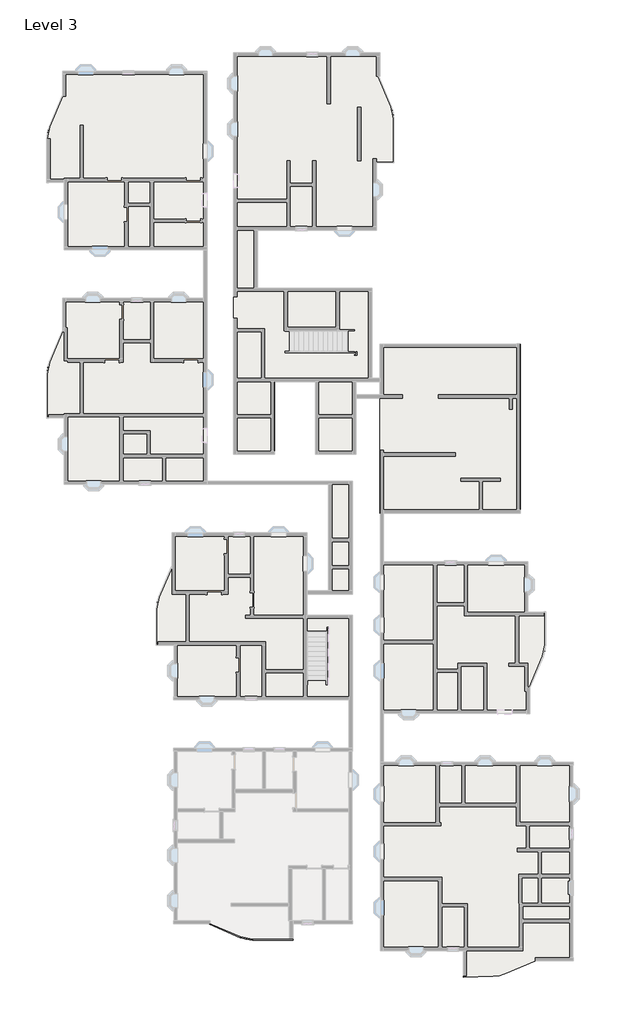
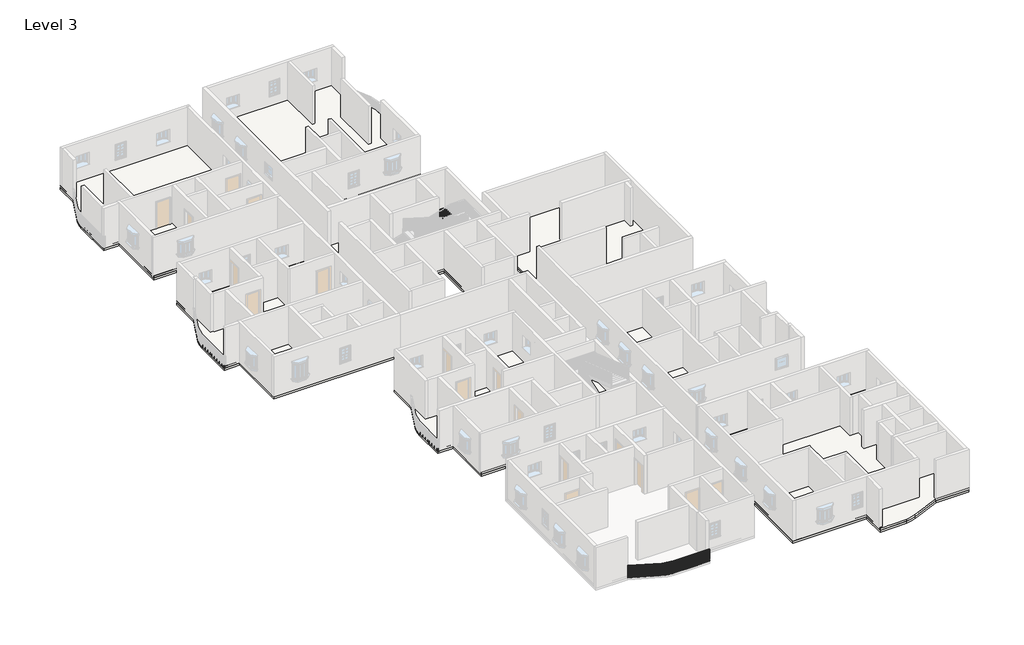
# One storey, part 5 of 14: 13 roofs, 12 slabs, 1 railing.
"""IFC4 building model written with IfcOpenShell, lengths in millimetres."""

from ifc_helpers import new_model, si_unit, point, frame, frame_2d, origin, place, context, project, spatial, polyline, circle_curve, trimmed, segment, composite_curve, outline, extrude, element, save
from ifc_brep_helpers import plane_surface, cylinder_surface, revolved_surface, advanced_brep

model = new_model("IFC4")

# Units and contexts
model_context = context("Model", 3, world=origin())
ifc_project = project(units=[si_unit("LENGTHUNIT", "METRE", prefix="MILLI")], contexts=[model_context])

# Site, building, storey
site = spatial("IfcSite", under=ifc_project)
building = spatial("IfcBuilding", under=site)
storey = spatial("IfcBuildingStorey", under=building, Name="Level 3", Elevation=6096.0)

# Railing
placement = place(None, origin())
element("IfcRailing", 1, ObjectType="Handrail - Rectangular", at=placement, inside=storey, context=model_context, shape_type="SolidModel", body=[
    advanced_brep(
    [(-10014.8722294, -25076.9923935, 7010.4), (-10014.8722294, -25076.9923935, 6959.6), (-10034.8694485, -25123.6909077, 6959.6), (-10034.8694485, -25123.6909077, 7010.4), (-8065.5370278, -25911.7359335, 7010.4), (-8065.5370278, -25911.7359335, 6959.6), (-8085.5342469, -25958.4344477, 6959.6), (-8085.5342469, -25958.4344477, 7010.4), (-7315.6413127, -26065.5416506, 6959.6), (-7315.6413127, -26065.5416506, 7010.4), (-7315.6413127, -26116.3416506, 6959.6), (-7315.6413127, -26116.3416506, 7010.4), (-4746.0891351, -26065.5416506, 7010.4), (-4746.0891351, -26116.3416506, 7010.4), (-4746.0891351, -26116.3416506, 6959.6), (-4746.0891351, -26065.5416506, 6959.6)],
    [
        (0, 1),
        (1, 2),
        (2, 3),
        (3, 0),
        (0, 4),
        (4, 5),
        (5, 1),
        (5, 6),
        (6, 2),
        (6, 7),
        (7, 3),
        (7, 4),
        (8, 5, circle_curve(frame((-7315.6413127, -24160.5416506, 6959.6), z_axis=(0.0, 0.0, -1.0), x_axis=(-0.3936460446736572, -0.9192620907623599, 0.0)), 1905.0)),
        (4, 9, circle_curve(frame((-7315.6413127, -24160.5416506, 7010.4), z_axis=(0.0, 0.0, 1.0), x_axis=(-0.3936460446736572, -0.9192620907623599, 0.0)), 1905.0)),
        (9, 8),
        (10, 6, circle_curve(frame((-7315.6413127, -24160.5416506, 6959.6), z_axis=(0.0, 0.0, -1.0), x_axis=(-0.3936460446736572, -0.9192620907623599, 0.0)), 1955.8)),
        (8, 10),
        (11, 7, circle_curve(frame((-7315.6413127, -24160.5416506, 7010.4), z_axis=(0.0, 0.0, -1.0), x_axis=(-0.3936460446736572, -0.9192620907623599, 0.0)), 1955.8)),
        (10, 11),
        (11, 9),
        (12, 13),
        (13, 14),
        (14, 15),
        (15, 12),
        (9, 12),
        (15, 8),
        (14, 10),
        (13, 11),
    ],
    [
        plane_surface(frame((-10024.8708389, -25100.3416506, 7010.4), z_axis=(-0.9192620907623597, 0.39364604467365766, 0.0), x_axis=(0.39364604467365766, 0.9192620907623597, 0.0))),
        plane_surface(frame((-10014.8722294, -25076.9923935, 7010.4), z_axis=(0.3936460446736571, 0.9192620907623599, 0.0), x_axis=(0.9192620907623599, -0.3936460446736571, 0.0))),
        plane_surface(frame((-10014.8722294, -25076.9923935, 6959.6), z_axis=(0.0, 0.0, -1.0), x_axis=(0.9192620907623599, -0.3936460446736571, 0.0))),
        plane_surface(frame((-10034.8694485, -25123.6909077, 6959.6), z_axis=(-0.3936460446736573, -0.9192620907623599, 0.0), x_axis=(0.9192620907623599, -0.3936460446736573, 0.0))),
        plane_surface(frame((-10034.8694485, -25123.6909077, 7010.4), z_axis=(0.0, 0.0, 1.0000000000000002), x_axis=(0.9192620907623599, -0.3936460446736573, 0.0))),
        revolved_surface(polyline([(-8065.537027803317, -25911.735933502296, 7010.4), (-8065.537027803317, -25911.735933502296, 6959.6)]), (-7315.6413127, -24160.5416506, 7010.4), (0.0, 0.0, 1.0)),
        plane_surface(frame((-7315.6413127, -24160.5416506, 6959.6), z_axis=(0.0, 0.0, -1.0), x_axis=(-0.3936460446736572, -0.9192620907623599, 0.0))),
        cylinder_surface(frame((-7315.6413127, -24160.5416506, 7010.4), z_axis=(0.0, 0.0, 1.0), x_axis=(-0.3936460446736572, -0.9192620907623599, 0.0)), 1955.8),
        plane_surface(frame((-7315.6413127, -24160.5416506, 7010.4), z_axis=(0.0, 0.0, 1.0), x_axis=(-0.3936460446736572, -0.9192620907623599, 0.0))),
        plane_surface(frame((-4746.0891351, -26090.9416506, 7010.4), z_axis=(1.0, 0.0, 0.0), x_axis=(0.0, 1.0, 0.0))),
        plane_surface(frame((-7315.6413127, -26065.5416506, 7010.4), z_axis=(0.0, 1.0, 0.0), x_axis=(1.0, 0.0, 0.0))),
        plane_surface(frame((-7315.6413127, -26065.5416506, 6959.6), z_axis=(0.0, 0.0, -1.0), x_axis=(1.0, 0.0, 0.0))),
        plane_surface(frame((-7315.6413127, -26116.3416506, 6959.6), z_axis=(0.0, -1.0, 0.0), x_axis=(1.0, 0.0, 0.0))),
        plane_surface(frame((-7315.6413127, -26116.3416506, 7010.4), z_axis=(0.0, 0.0, 1.0), x_axis=(1.0, 0.0, 0.0))),
    ],
    [
        (0, [[1, 2, 3, 4]]),
        (1, [[-1, 5, 6, 7]]),
        (2, [[-2, -7, 8, 9]]),
        (3, [[-3, -9, 10, 11]]),
        (4, [[-4, -11, 12, -5]]),
        (5, [[13, -6, 14, 15]]),
        (6, [[16, -8, -13, 17]]),
        (7, [[18, -10, -16, 19]]),
        (8, [[-14, -12, -18, 20]]),
        (9, [[21, 22, 23, 24]]),
        (10, [[-15, 25, -24, 26]]),
        (11, [[-17, -26, -23, 27]]),
        (12, [[-19, -27, -22, 28]]),
        (13, [[-20, -28, -21, -25]]),
    ],
),
    extrude(outline(polyline([(-4785.1663127, -26100.4666506), (-4785.1663127, -26081.4166506), (-4766.1163127, -26081.4166506), (-4766.1163127, -26100.4666506), (-4785.1663127, -26100.4666506)])), frame((0.0, 0.0, 6096.0), z_axis=(0.0, 0.0, 1.0), x_axis=(1.0, 0.0, 0.0)), (0.0, 0.0, 1.0), 863.6),
    extrude(outline(polyline([(-4886.7663127, -26100.4666506), (-4886.7663127, -26081.4166506), (-4867.7163127, -26081.4166506), (-4867.7163127, -26100.4666506), (-4886.7663127, -26100.4666506)])), frame((0.0, 0.0, 6096.0), z_axis=(0.0, 0.0, 1.0), x_axis=(1.0, 0.0, 0.0)), (0.0, 0.0, 1.0), 863.6),
    extrude(outline(polyline([(-4988.3663127, -26100.4666506), (-4988.3663127, -26081.4166506), (-4969.3163127, -26081.4166506), (-4969.3163127, -26100.4666506), (-4988.3663127, -26100.4666506)])), frame((0.0, 0.0, 6096.0), z_axis=(0.0, 0.0, 1.0), x_axis=(1.0, 0.0, 0.0)), (0.0, 0.0, 1.0), 863.6),
    extrude(outline(polyline([(-5089.9663127, -26100.4666506), (-5089.9663127, -26081.4166506), (-5070.9163127, -26081.4166506), (-5070.9163127, -26100.4666506), (-5089.9663127, -26100.4666506)])), frame((0.0, 0.0, 6096.0), z_axis=(0.0, 0.0, 1.0), x_axis=(1.0, 0.0, 0.0)), (0.0, 0.0, 1.0), 863.6),
    extrude(outline(polyline([(-5191.5663127, -26100.4666506), (-5191.5663127, -26081.4166506), (-5172.5163127, -26081.4166506), (-5172.5163127, -26100.4666506), (-5191.5663127, -26100.4666506)])), frame((0.0, 0.0, 6096.0), z_axis=(0.0, 0.0, 1.0), x_axis=(1.0, 0.0, 0.0)), (0.0, 0.0, 1.0), 863.6),
    extrude(outline(polyline([(-5293.1663127, -26100.4666506), (-5293.1663127, -26081.4166506), (-5274.1163127, -26081.4166506), (-5274.1163127, -26100.4666506), (-5293.1663127, -26100.4666506)])), frame((0.0, 0.0, 6096.0), z_axis=(0.0, 0.0, 1.0), x_axis=(1.0, 0.0, 0.0)), (0.0, 0.0, 1.0), 863.6),
    extrude(outline(polyline([(-5394.7663127, -26100.4666506), (-5394.7663127, -26081.4166506), (-5375.7163127, -26081.4166506), (-5375.7163127, -26100.4666506), (-5394.7663127, -26100.4666506)])), frame((0.0, 0.0, 6096.0), z_axis=(0.0, 0.0, 1.0), x_axis=(1.0, 0.0, 0.0)), (0.0, 0.0, 1.0), 863.6),
    extrude(outline(polyline([(-5496.3663127, -26100.4666506), (-5496.3663127, -26081.4166506), (-5477.3163127, -26081.4166506), (-5477.3163127, -26100.4666506), (-5496.3663127, -26100.4666506)])), frame((0.0, 0.0, 6096.0), z_axis=(0.0, 0.0, 1.0), x_axis=(1.0, 0.0, 0.0)), (0.0, 0.0, 1.0), 863.6),
    extrude(outline(polyline([(-5597.9663127, -26100.4666506), (-5597.9663127, -26081.4166506), (-5578.9163127, -26081.4166506), (-5578.9163127, -26100.4666506), (-5597.9663127, -26100.4666506)])), frame((0.0, 0.0, 6096.0), z_axis=(0.0, 0.0, 1.0), x_axis=(1.0, 0.0, 0.0)), (0.0, 0.0, 1.0), 863.6),
    extrude(outline(polyline([(-5699.5663127, -26100.4666506), (-5699.5663127, -26081.4166506), (-5680.5163127, -26081.4166506), (-5680.5163127, -26100.4666506), (-5699.5663127, -26100.4666506)])), frame((0.0, 0.0, 6096.0), z_axis=(0.0, 0.0, 1.0), x_axis=(1.0, 0.0, 0.0)), (0.0, 0.0, 1.0), 863.6),
    extrude(outline(polyline([(-5801.1663127, -26100.4666506), (-5801.1663127, -26081.4166506), (-5782.1163127, -26081.4166506), (-5782.1163127, -26100.4666506), (-5801.1663127, -26100.4666506)])), frame((0.0, 0.0, 6096.0), z_axis=(0.0, 0.0, 1.0), x_axis=(1.0, 0.0, 0.0)), (0.0, 0.0, 1.0), 863.6),
    extrude(outline(polyline([(-5902.7663127, -26100.4666506), (-5902.7663127, -26081.4166506), (-5883.7163127, -26081.4166506), (-5883.7163127, -26100.4666506), (-5902.7663127, -26100.4666506)])), frame((0.0, 0.0, 6096.0), z_axis=(0.0, 0.0, 1.0), x_axis=(1.0, 0.0, 0.0)), (0.0, 0.0, 1.0), 863.6),
    extrude(outline(polyline([(-6004.3663127, -26100.4666506), (-6004.3663127, -26081.4166506), (-5985.3163127, -26081.4166506), (-5985.3163127, -26100.4666506), (-6004.3663127, -26100.4666506)])), frame((0.0, 0.0, 6096.0), z_axis=(0.0, 0.0, 1.0), x_axis=(1.0, 0.0, 0.0)), (0.0, 0.0, 1.0), 863.6),
    extrude(outline(polyline([(-6105.9663127, -26100.4666506), (-6105.9663127, -26081.4166506), (-6086.9163127, -26081.4166506), (-6086.9163127, -26100.4666506), (-6105.9663127, -26100.4666506)])), frame((0.0, 0.0, 6096.0), z_axis=(0.0, 0.0, 1.0), x_axis=(1.0, 0.0, 0.0)), (0.0, 0.0, 1.0), 863.6),
    extrude(outline(polyline([(-6207.5663127, -26100.4666506), (-6207.5663127, -26081.4166506), (-6188.5163127, -26081.4166506), (-6188.5163127, -26100.4666506), (-6207.5663127, -26100.4666506)])), frame((0.0, 0.0, 6096.0), z_axis=(0.0, 0.0, 1.0), x_axis=(1.0, 0.0, 0.0)), (0.0, 0.0, 1.0), 863.6),
    extrude(outline(polyline([(-6309.1663127, -26100.4666506), (-6309.1663127, -26081.4166506), (-6290.1163127, -26081.4166506), (-6290.1163127, -26100.4666506), (-6309.1663127, -26100.4666506)])), frame((0.0, 0.0, 6096.0), z_axis=(0.0, 0.0, 1.0), x_axis=(1.0, 0.0, 0.0)), (0.0, 0.0, 1.0), 863.6),
    extrude(outline(polyline([(-6410.7663127, -26100.4666506), (-6410.7663127, -26081.4166506), (-6391.7163127, -26081.4166506), (-6391.7163127, -26100.4666506), (-6410.7663127, -26100.4666506)])), frame((0.0, 0.0, 6096.0), z_axis=(0.0, 0.0, 1.0), x_axis=(1.0, 0.0, 0.0)), (0.0, 0.0, 1.0), 863.6),
    extrude(outline(polyline([(-6512.3663127, -26100.4666506), (-6512.3663127, -26081.4166506), (-6493.3163127, -26081.4166506), (-6493.3163127, -26100.4666506), (-6512.3663127, -26100.4666506)])), frame((0.0, 0.0, 6096.0), z_axis=(0.0, 0.0, 1.0), x_axis=(1.0, 0.0, 0.0)), (0.0, 0.0, 1.0), 863.6),
    extrude(outline(polyline([(-6613.9663127, -26100.4666506), (-6613.9663127, -26081.4166506), (-6594.9163127, -26081.4166506), (-6594.9163127, -26100.4666506), (-6613.9663127, -26100.4666506)])), frame((0.0, 0.0, 6096.0), z_axis=(0.0, 0.0, 1.0), x_axis=(1.0, 0.0, 0.0)), (0.0, 0.0, 1.0), 863.6),
    extrude(outline(polyline([(-6715.5663127, -26100.4666506), (-6715.5663127, -26081.4166506), (-6696.5163127, -26081.4166506), (-6696.5163127, -26100.4666506), (-6715.5663127, -26100.4666506)])), frame((0.0, 0.0, 6096.0), z_axis=(0.0, 0.0, 1.0), x_axis=(1.0, 0.0, 0.0)), (0.0, 0.0, 1.0), 863.6),
    extrude(outline(polyline([(-6817.1663127, -26100.4666506), (-6817.1663127, -26081.4166506), (-6798.1163127, -26081.4166506), (-6798.1163127, -26100.4666506), (-6817.1663127, -26100.4666506)])), frame((0.0, 0.0, 6096.0), z_axis=(0.0, 0.0, 1.0), x_axis=(1.0, 0.0, 0.0)), (0.0, 0.0, 1.0), 863.6),
    extrude(outline(polyline([(-6918.7663127, -26100.4666506), (-6918.7663127, -26081.4166506), (-6899.7163127, -26081.4166506), (-6899.7163127, -26100.4666506), (-6918.7663127, -26100.4666506)])), frame((0.0, 0.0, 6096.0), z_axis=(0.0, 0.0, 1.0), x_axis=(1.0, 0.0, 0.0)), (0.0, 0.0, 1.0), 863.6),
    extrude(outline(polyline([(-7020.3663127, -26100.4666506), (-7020.3663127, -26081.4166506), (-7001.3163127, -26081.4166506), (-7001.3163127, -26100.4666506), (-7020.3663127, -26100.4666506)])), frame((0.0, 0.0, 6096.0), z_axis=(0.0, 0.0, 1.0), x_axis=(1.0, 0.0, 0.0)), (0.0, 0.0, 1.0), 863.6),
    extrude(outline(polyline([(-7121.9663127, -26100.4666506), (-7121.9663127, -26081.4166506), (-7102.9163127, -26081.4166506), (-7102.9163127, -26100.4666506), (-7121.9663127, -26100.4666506)])), frame((0.0, 0.0, 6096.0), z_axis=(0.0, 0.0, 1.0), x_axis=(1.0, 0.0, 0.0)), (0.0, 0.0, 1.0), 863.6),
    extrude(outline(polyline([(-7223.5663127, -26100.4666506), (-7223.5663127, -26081.4166506), (-7204.5163127, -26081.4166506), (-7204.5163127, -26100.4666506), (-7223.5663127, -26100.4666506)])), frame((0.0, 0.0, 6096.0), z_axis=(0.0, 0.0, 1.0), x_axis=(1.0, 0.0, 0.0)), (0.0, 0.0, 1.0), 863.6),
    extrude(outline(polyline([(-7395.3185803, -26098.8530973), (-7394.6296262, -26079.8155596), (-7375.5920885, -26080.5045137), (-7376.2810426, -26099.5420514), (-7395.3185803, -26098.8530973)])), frame((0.0, 0.0, 6096.0), z_axis=(0.0, 0.0, 1.0), x_axis=(1.0, 0.0, 0.0)), (0.0, 0.0, 1.0), 863.6),
    extrude(outline(polyline([(-7497.177549, -26091.9774704), (-7495.4880357, -26073.0025384), (-7476.5131037, -26074.6920517), (-7478.2026169, -26093.6669837), (-7497.177549, -26091.9774704)])), frame((0.0, 0.0, 6096.0), z_axis=(0.0, 0.0, 1.0), x_axis=(1.0, 0.0, 0.0)), (0.0, 0.0, 1.0), 863.6),
    extrude(outline(polyline([(-7598.5337632, -26079.7528408), (-7595.8483698, -26060.8930645), (-7576.9885935, -26063.5784579), (-7579.6739869, -26082.4382342), (-7598.5337632, -26079.7528408)])), frame((0.0, 0.0, 6096.0), z_axis=(0.0, 0.0, 1.0), x_axis=(1.0, 0.0, 0.0)), (0.0, 0.0, 1.0), 863.6),
    extrude(outline(polyline([(-7699.1065227, -26062.2130639), (-7695.4326862, -26043.5206744), (-7676.7402967, -26047.1945108), (-7680.4141332, -26065.8869003), (-7699.1065227, -26062.2130639)])), frame((0.0, 0.0, 6096.0), z_axis=(0.0, 0.0, 1.0), x_axis=(1.0, 0.0, 0.0)), (0.0, 0.0, 1.0), 863.6),
    extrude(outline(polyline([(-7798.6172969, -26039.4067149), (-7793.9651918, -26020.9334797), (-7775.4919566, -26025.5855848), (-7780.1440617, -26044.05882), (-7798.6172969, -26039.4067149)])), frame((0.0, 0.0, 6096.0), z_axis=(0.0, 0.0, 1.0), x_axis=(1.0, 0.0, 0.0)), (0.0, 0.0, 1.0), 863.6),
    extrude(outline(polyline([(-7896.7904963, -26011.396955), (-7891.1730064, -25993.1940347), (-7872.9700861, -25998.8115246), (-7878.587576, -26017.0144449), (-7896.7904963, -26011.396955)])), frame((0.0, 0.0, 6096.0), z_axis=(0.0, 0.0, 1.0), x_axis=(1.0, 0.0, 0.0)), (0.0, 0.0, 1.0), 863.6),
    extrude(outline(polyline([(-7993.3542357, -25978.2613554), (-7986.7869183, -25960.379162), (-7968.9047249, -25966.9464794), (-7975.4720423, -25984.8286729), (-7993.3542357, -25978.2613554)])), frame((0.0, 0.0, 6096.0), z_axis=(0.0, 0.0, 1.0), x_axis=(1.0, 0.0, 0.0)), (0.0, 0.0, 1.0), 863.6),
    extrude(outline(polyline([(-8169.4357205, -25905.2369062), (-8161.9367633, -25887.7249634), (-8144.4248205, -25895.2239205), (-8151.9237777, -25912.7358634), (-8169.4357205, -25905.2369062)])), frame((0.0, 0.0, 6096.0), z_axis=(0.0, 0.0, 1.0), x_axis=(1.0, 0.0, 0.0)), (0.0, 0.0, 1.0), 863.6),
    extrude(outline(polyline([(-8262.8327489, -25865.2424681), (-8255.3337918, -25847.7305252), (-8237.8218489, -25855.2294824), (-8245.3208061, -25872.7414252), (-8262.8327489, -25865.2424681)])), frame((0.0, 0.0, 6096.0), z_axis=(0.0, 0.0, 1.0), x_axis=(1.0, 0.0, 0.0)), (0.0, 0.0, 1.0), 863.6),
    extrude(outline(polyline([(-8356.2297773, -25825.2480299), (-8348.7308202, -25807.7360871), (-8331.2188774, -25815.2350443), (-8338.7178345, -25832.7469871), (-8356.2297773, -25825.2480299)])), frame((0.0, 0.0, 6096.0), z_axis=(0.0, 0.0, 1.0), x_axis=(1.0, 0.0, 0.0)), (0.0, 0.0, 1.0), 863.6),
    extrude(outline(polyline([(-8449.6268058, -25785.2535918), (-8442.1278486, -25767.741649), (-8424.6159058, -25775.2406061), (-8432.1148629, -25792.752549), (-8449.6268058, -25785.2535918)])), frame((0.0, 0.0, 6096.0), z_axis=(0.0, 0.0, 1.0), x_axis=(1.0, 0.0, 0.0)), (0.0, 0.0, 1.0), 863.6),
    extrude(outline(polyline([(-8543.0238342, -25745.2591537), (-8535.524877, -25727.7472108), (-8518.0129342, -25735.246168), (-8525.5118914, -25752.7581108), (-8543.0238342, -25745.2591537)])), frame((0.0, 0.0, 6096.0), z_axis=(0.0, 0.0, 1.0), x_axis=(1.0, 0.0, 0.0)), (0.0, 0.0, 1.0), 863.6),
    extrude(outline(polyline([(-8636.4208626, -25705.2647155), (-8628.9219055, -25687.7527727), (-8611.4099626, -25695.2517298), (-8618.9089198, -25712.7636727), (-8636.4208626, -25705.2647155)])), frame((0.0, 0.0, 6096.0), z_axis=(0.0, 0.0, 1.0), x_axis=(1.0, 0.0, 0.0)), (0.0, 0.0, 1.0), 863.6),
    extrude(outline(polyline([(-8729.817891, -25665.2702774), (-8722.3189339, -25647.7583346), (-8704.806991, -25655.2572917), (-8712.3059482, -25672.7692345), (-8729.817891, -25665.2702774)])), frame((0.0, 0.0, 6096.0), z_axis=(0.0, 0.0, 1.0), x_axis=(1.0, 0.0, 0.0)), (0.0, 0.0, 1.0), 863.6),
    extrude(outline(polyline([(-8823.2149194, -25625.2758392), (-8815.7159623, -25607.7638964), (-8798.2040195, -25615.2628536), (-8805.7029766, -25632.7747964), (-8823.2149194, -25625.2758392)])), frame((0.0, 0.0, 6096.0), z_axis=(0.0, 0.0, 1.0), x_axis=(1.0, 0.0, 0.0)), (0.0, 0.0, 1.0), 863.6),
    extrude(outline(polyline([(-8916.6119479, -25585.2814011), (-8909.1129907, -25567.7694583), (-8891.6010479, -25575.2684154), (-8899.100005, -25592.7803583), (-8916.6119479, -25585.2814011)])), frame((0.0, 0.0, 6096.0), z_axis=(0.0, 0.0, 1.0), x_axis=(1.0, 0.0, 0.0)), (0.0, 0.0, 1.0), 863.6),
    extrude(outline(polyline([(-9010.0089763, -25545.286963), (-9002.5100191, -25527.7750201), (-8984.9980763, -25535.2739773), (-8992.4970335, -25552.7859201), (-9010.0089763, -25545.286963)])), frame((0.0, 0.0, 6096.0), z_axis=(0.0, 0.0, 1.0), x_axis=(1.0, 0.0, 0.0)), (0.0, 0.0, 1.0), 863.6),
    extrude(outline(polyline([(-9103.4060047, -25505.2925248), (-9095.9070476, -25487.780582), (-9078.3951047, -25495.2795391), (-9085.8940619, -25512.791482), (-9103.4060047, -25505.2925248)])), frame((0.0, 0.0, 6096.0), z_axis=(0.0, 0.0, 1.0), x_axis=(1.0, 0.0, 0.0)), (0.0, 0.0, 1.0), 863.6),
    extrude(outline(polyline([(-9196.8030331, -25465.2980867), (-9189.304076, -25447.7861439), (-9171.7921332, -25455.285101), (-9179.2910903, -25472.7970438), (-9196.8030331, -25465.2980867)])), frame((0.0, 0.0, 6096.0), z_axis=(0.0, 0.0, 1.0), x_axis=(1.0, 0.0, 0.0)), (0.0, 0.0, 1.0), 863.6),
    extrude(outline(polyline([(-9290.2000616, -25425.3036485), (-9282.7011044, -25407.7917057), (-9265.1891616, -25415.2906629), (-9272.6881187, -25432.8026057), (-9290.2000616, -25425.3036485)])), frame((0.0, 0.0, 6096.0), z_axis=(0.0, 0.0, 1.0), x_axis=(1.0, 0.0, 0.0)), (0.0, 0.0, 1.0), 863.6),
    extrude(outline(polyline([(-9383.59709, -25385.3092104), (-9376.0981328, -25367.7972676), (-9358.58619, -25375.2962247), (-9366.0851471, -25392.8081676), (-9383.59709, -25385.3092104)])), frame((0.0, 0.0, 6096.0), z_axis=(0.0, 0.0, 1.0), x_axis=(1.0, 0.0, 0.0)), (0.0, 0.0, 1.0), 863.6),
    extrude(outline(polyline([(-9476.9941184, -25345.3147723), (-9469.4951612, -25327.8028294), (-9451.9832184, -25335.3017866), (-9459.4821756, -25352.8137294), (-9476.9941184, -25345.3147723)])), frame((0.0, 0.0, 6096.0), z_axis=(0.0, 0.0, 1.0), x_axis=(1.0, 0.0, 0.0)), (0.0, 0.0, 1.0), 863.6),
    extrude(outline(polyline([(-9570.3911468, -25305.3203341), (-9562.8921897, -25287.8083913), (-9545.3802468, -25295.3073485), (-9552.879204, -25312.8192913), (-9570.3911468, -25305.3203341)])), frame((0.0, 0.0, 6096.0), z_axis=(0.0, 0.0, 1.0), x_axis=(1.0, 0.0, 0.0)), (0.0, 0.0, 1.0), 863.6),
    extrude(outline(polyline([(-9663.7881752, -25265.325896), (-9656.2892181, -25247.8139532), (-9638.7772753, -25255.3129103), (-9646.2762324, -25272.8248531), (-9663.7881752, -25265.325896)])), frame((0.0, 0.0, 6096.0), z_axis=(0.0, 0.0, 1.0), x_axis=(1.0, 0.0, 0.0)), (0.0, 0.0, 1.0), 863.6),
    extrude(outline(polyline([(-9757.1852037, -25225.3314579), (-9749.6862465, -25207.819515), (-9732.1743037, -25215.3184722), (-9739.6732608, -25232.830415), (-9757.1852037, -25225.3314579)])), frame((0.0, 0.0, 6096.0), z_axis=(0.0, 0.0, 1.0), x_axis=(1.0, 0.0, 0.0)), (0.0, 0.0, 1.0), 863.6),
    extrude(outline(polyline([(-9850.5822321, -25185.3370197), (-9843.0832749, -25167.8250769), (-9825.5713321, -25175.324034), (-9833.0702893, -25192.8359769), (-9850.5822321, -25185.3370197)])), frame((0.0, 0.0, 6096.0), z_axis=(0.0, 0.0, 1.0), x_axis=(1.0, 0.0, 0.0)), (0.0, 0.0, 1.0), 863.6),
    extrude(outline(polyline([(-9943.9792605, -25145.3425816), (-9936.4803034, -25127.8306387), (-9918.9683605, -25135.3295959), (-9926.4673177, -25152.8415387), (-9943.9792605, -25145.3425816)])), frame((0.0, 0.0, 6096.0), z_axis=(0.0, 0.0, 1.0), x_axis=(1.0, 0.0, 0.0)), (0.0, 0.0, 1.0), 863.6),
    extrude(outline(polyline([(-7325.1663127, -26100.4666506), (-7325.1663127, -26081.4166506), (-7306.1163127, -26081.4166506), (-7306.1163127, -26100.4666506), (-7325.1663127, -26100.4666506)])), frame((0.0, 0.0, 6096.0), z_axis=(0.0, 0.0, 1.0), x_axis=(1.0, 0.0, 0.0)), (0.0, 0.0, 1.0), 863.6),
    extrude(outline(polyline([(-8088.0410874, -25940.0916834), (-8080.5421302, -25922.5797406), (-8063.0301874, -25930.0786978), (-8070.5291445, -25947.5906406), (-8088.0410874, -25940.0916834)])), frame((0.0, 0.0, 6096.0), z_axis=(0.0, 0.0, 1.0), x_axis=(1.0, 0.0, 0.0)), (0.0, 0.0, 1.0), 863.6),
    extrude(outline(polyline([(-4765.1391351, -26100.4666506), (-4765.1391351, -26081.4166506), (-4746.0891351, -26081.4166506), (-4746.0891351, -26100.4666506), (-4765.1391351, -26100.4666506)])), frame((0.0, 0.0, 6096.0), z_axis=(0.0, 0.0, 1.0), x_axis=(1.0, 0.0, 0.0)), (0.0, 0.0, 1.0), 863.6),
    extrude(outline(polyline([(-10028.6203175, -25109.097622), (-10021.1213604, -25091.5856792), (-10003.6094175, -25099.0846363), (-10011.1083747, -25116.5965792), (-10028.6203175, -25109.097622)])), frame((0.0, 0.0, 6096.0), z_axis=(0.0, 0.0, 1.0), x_axis=(1.0, 0.0, 0.0)), (0.0, 0.0, 1.0), 863.6),
])

# Roofs
element("IfcRoof", 2, ObjectType="Generic - 12\"", at=placement, inside=storey, context=model_context, shape_type="SweptSolid", body=[
    extrude(outline(composite_curve([segment(polyline([(6070.4380523, -26783.9042694), (812.6380523, -26783.9042694), (812.6380523, -14845.9042694), (13017.3380523, -14845.9042694), (13017.3380523, -27431.6042694), (10660.5280667, -27431.6042694), (8711.1928652, -28266.3478094)]), True, "CONTINUOUS"), segment(trimmed(circle_curve(frame_2d((7951.2985405, -26491.8042694)), 1930.4), [point((8711.1928652, -28266.3478094))], [point((7953.0959373, -28422.2034326))], False, "CARTESIAN"), True, "CONTINUOUS"), segment(polyline([(7953.0959373, -28422.2034326), (6070.4380523, -28487.9472947), (6070.4380523, -26783.9042694)]), True, "CONTINUOUS")], self_intersect=False)), frame((0.0, 0.0, 6096.0), z_axis=(0.0, 0.0, 1.0), x_axis=(1.0, 0.0, 0.0)), (0.0, 0.0, 1.0), 152.4),
])
element("IfcRoof", 3, ObjectType="Generic - 12\"", at=placement, inside=storey, context=model_context, shape_type="SweptSolid", body=[
    extrude(outline(composite_curve([segment(polyline([(10274.1380523, -11759.8042694), (803.8108649, -11759.8042694), (803.8108649, -2133.2042694), (10159.8380523, -2133.2042694), (10159.8380523, -5352.6542694), (11264.7380523, -5352.6542694), (11264.7380523, -7397.5810633)]), True, "CONTINUOUS"), segment(trimmed(circle_curve(frame_2d((9334.3380523, -7397.5810633)), 1930.4), [point((11264.7380523, -7397.5810633))], [point((11108.8815923, -8157.475388))], False, "CARTESIAN"), True, "CONTINUOUS"), segment(polyline([(11108.8815923, -8157.475388), (10274.1380523, -10106.8105895), (10274.1380523, -11759.8042694)]), True, "CONTINUOUS")], self_intersect=False)), frame((0.0, 0.0, 6096.0), z_axis=(0.0, 0.0, 1.0), x_axis=(1.0, 0.0, 0.0)), (0.0, 0.0, 1.0), 152.4),
])
element("IfcRoof", 4, ObjectType="Generic - 12\"", at=placement, inside=storey, context=model_context, shape_type="SweptSolid", body=[
    extrude(outline(composite_curve([segment(polyline([(-13395.387215, -7421.9416506), (-13395.387215, -5140.4900045)]), True, "CONTINUOUS"), segment(trimmed(circle_curve(frame_2d((-11464.987215, -5140.4900045)), 1930.4), [point((-13395.387215, -5140.4900045))], [point((-13239.530755, -4380.5956799))], False, "CARTESIAN"), True, "CONTINUOUS"), segment(polyline([(-13239.530755, -4380.5956799), (-12404.787215, -2431.2604783), (-12404.787215, -322.6416506), (-3857.687215, -322.6416506), (-3857.687215, -5523.2916506), (-974.1891351, -5523.2916506), (-974.1891351, -10889.0416506), (-12290.487215, -10889.0416506), (-12290.487215, -7421.9416506), (-13395.387215, -7421.9416506)]), True, "CONTINUOUS")], self_intersect=False)), frame((0.0, 0.0, 6096.0), z_axis=(0.0, 0.0, 1.0), x_axis=(1.0, 0.0, 0.0)), (0.0, 0.0, 1.0), 152.4),
])
element("IfcRoof", 5, ObjectType="Generic - 12\"", at=placement, inside=storey, context=model_context, shape_type="SweptSolid", body=[
    extrude(outline(polyline([(-2472.7891351, 2953.9583494), (-961.4891351, 2953.9583494), (-961.4891351, -4202.4916506), (-2472.7891351, -4202.4916506), (-2472.7891351, 2953.9583494)])), frame((0.0, 0.0, 6096.0), z_axis=(0.0, 0.0, 1.0), x_axis=(1.0, 0.0, 0.0)), (0.0, 0.0, 1.0), 152.4),
])
element("IfcRoof", 6, ObjectType="Generic - 12\"", at=placement, inside=storey, context=model_context, shape_type="SweptSolid", body=[
    extrude(outline(composite_curve([segment(polyline([(-10194.3891351, 2750.7583494), (-19236.7891351, 2750.7583494), (-19236.7891351, 6979.8583494), (-20341.6891351, 6979.8583494), (-20341.6891351, 9746.7948172)]), True, "CONTINUOUS"), segment(trimmed(circle_curve(frame_2d((-18411.2891351, 9746.7948172)), 1930.4), [point((-20341.6891351, 9746.7948172))], [point((-20185.8326751, 10506.6891419))], False, "CARTESIAN"), True, "CONTINUOUS"), segment(polyline([(-20185.8326751, 10506.6891419), (-19351.0891351, 12456.0243434), (-19351.0891351, 14536.3583494), (-10194.3891351, 14536.3583494), (-10194.3891351, 2750.7583494)]), True, "CONTINUOUS")], self_intersect=False)), frame((0.0, 0.0, 6096.0), z_axis=(0.0, 0.0, 1.0), x_axis=(1.0, 0.0, 0.0)), (0.0, 0.0, 1.0), 152.4),
])
element("IfcRoof", 7, ObjectType="Generic - 12\"", at=placement, inside=storey, context=model_context, shape_type="SweptSolid", body=[
    extrude(outline(composite_curve([segment(polyline([(-10194.3891351, 17609.7583494), (-19236.7891351, 17609.7583494), (-19236.7891351, 21889.6583494), (-20341.6891351, 21889.6583494), (-20341.6891351, 24656.5948172)]), True, "CONTINUOUS"), segment(trimmed(circle_curve(frame_2d((-18411.2891351, 24656.5948172)), 1930.4), [point((-20341.6891351, 24656.5948172))], [point((-20185.8326751, 25416.4891419))], False, "CARTESIAN"), True, "CONTINUOUS"), segment(polyline([(-20185.8326751, 25416.4891419), (-19351.0891351, 27365.8243434), (-19351.0891351, 28950.8583494), (-10194.3891351, 28950.8583494), (-10194.3891351, 17609.7583494)]), True, "CONTINUOUS")], self_intersect=False)), frame((0.0, 0.0, 6096.0), z_axis=(0.0, 0.0, 1.0), x_axis=(1.0, 0.0, 0.0)), (0.0, 0.0, 1.0), 152.4),
])
element("IfcRoof", 8, ObjectType="Generic - 12\"", at=placement, inside=storey, context=model_context, shape_type="SweptSolid", body=[
    extrude(outline(composite_curve([segment(polyline([(-8492.5891351, 18875.1215905), (-8492.5891351, 30101.9215905), (664.1108649, 30101.9215905), (664.1108649, 28631.1875845), (1498.8544049, 26681.8523829)]), True, "CONTINUOUS"), segment(trimmed(circle_curve(frame_2d((-275.6891351, 25921.9580583)), 1930.4), [point((1498.8544049, 26681.8523829))], [point((1654.7108649, 25921.9580583))], False, "CARTESIAN"), True, "CONTINUOUS"), segment(polyline([(1654.7108649, 25921.9580583), (1654.7108649, 23155.0215905), (549.8108649, 23155.0215905), (549.8108649, 18875.1215905), (-8492.5891351, 18875.1215905)]), True, "CONTINUOUS")], self_intersect=False)), frame((0.0, 0.0, 6096.0), z_axis=(0.0, 0.0, 1.0), x_axis=(1.0, 0.0, 0.0)), (0.0, 0.0, 1.0), 152.4),
])
element("IfcRoof", 9, ObjectType="Generic - 12\"", at=placement, inside=storey, context=model_context, shape_type="SweptSolid", body=[
    extrude(outline(polyline([(-8492.5891351, 9478.4949943), (-5914.4891351, 9478.4949943), (-5914.4891351, 4665.1949943), (-8492.5891351, 4665.1949943), (-8492.5891351, 9478.4949943)])), frame((0.0, 0.0, 6096.0), z_axis=(0.0, 0.0, 1.0), x_axis=(1.0, 0.0, 0.0)), (0.0, 0.0, 1.0), 152.4),
])
element("IfcRoof", 10, ObjectType="Generic - 12\"", at=placement, inside=storey, context=model_context, shape_type="SweptSolid", body=[
    extrude(outline(polyline([(-3310.9891351, 9478.4949943), (-745.5891351, 9478.4949943), (-745.5891351, 4652.4949943), (-3310.9891351, 4652.4949943), (-3310.9891351, 9478.4949943)])), frame((0.0, 0.0, 6096.0), z_axis=(0.0, 0.0, 1.0), x_axis=(1.0, 0.0, 0.0)), (0.0, 0.0, 1.0), 152.4),
])
element("IfcRoof", 11, ObjectType="Generic - 12\"", at=placement, inside=storey, context=model_context, shape_type="SweptSolid", body=[
    extrude(outline(polyline([(-8492.5891351, 19078.3215905), (-6993.9891351, 19078.3215905), (-6993.9891351, 14988.9215905), (-8492.5891351, 14988.9215905), (-8492.5891351, 19078.3215905)])), frame((0.0, 0.0, 6096.0), z_axis=(0.0, 0.0, 1.0), x_axis=(1.0, 0.0, 0.0)), (0.0, 0.0, 1.0), 152.4),
])
element("IfcRoof", 12, ObjectType="Generic - 12\"", at=placement, inside=storey, context=model_context, shape_type="SweptSolid", body=[
    extrude(outline(polyline([(-8492.5891351, 15192.1215905), (257.7108649, 15192.1215905), (257.7108649, 9275.2949943), (-8492.5891351, 9275.2949943), (-8492.5891351, 15192.1215905)])), frame((0.0, 0.0, 6096.0), z_axis=(0.0, 0.0, 1.0), x_axis=(1.0, 0.0, 0.0)), (0.0, 0.0, 1.0), 152.4),
])
element("IfcRoof", 13, ObjectType="Generic - 12\"", at=placement, inside=storey, context=model_context, shape_type="SweptSolid", body=[
    extrude(outline(polyline([(793.5880523, 11646.2957306), (9677.2380523, 11646.2957306), (9677.2380523, 940.1957306), (793.5880523, 940.1957306), (793.5880523, 11646.2957306)])), frame((0.0, 0.0, 6096.0), z_axis=(0.0, 0.0, 1.0), x_axis=(1.0, 0.0, 0.0)), (0.0, 0.0, 1.0), 152.4),
])
element("IfcRoof", 14, ObjectType="Generic - 12\"", at=placement, inside=storey, context=model_context, shape_type="SweptSolid", body=[
    extrude(outline(composite_curve([segment(polyline([(-8492.5891351, 18875.1215905), (-8492.5891351, 30101.9215905), (664.1108649, 30101.9215905), (664.1108649, 28631.1875845), (1498.8544049, 26681.8523829)]), True, "CONTINUOUS"), segment(trimmed(circle_curve(frame_2d((-275.6891351, 25921.9580583)), 1930.4), [point((1498.8544049, 26681.8523829))], [point((1654.7108649, 25921.9580583))], False, "CARTESIAN"), True, "CONTINUOUS"), segment(polyline([(1654.7108649, 25921.9580583), (1654.7108649, 23155.0215905), (549.8108649, 23155.0215905), (549.8108649, 18875.1215905), (-8492.5891351, 18875.1215905)]), True, "CONTINUOUS")], self_intersect=False)), frame((0.0, 0.0, 6096.0), z_axis=(0.0, 0.0, 1.0), x_axis=(1.0, 0.0, 0.0)), (0.0, 0.0, 1.0), 152.4),
])

# Slabs
element("IfcSlab", 15, ObjectType="Generic - 12\"", at=placement, inside=storey, context=model_context, shape_type="SweptSolid", body=[
    extrude(outline(composite_curve([segment(polyline([(-20341.6891351, 21889.6583494), (-20341.6891351, 24656.5948172)]), True, "CONTINUOUS"), segment(trimmed(circle_curve(frame_2d((-18411.2891351, 24656.5948172)), 1930.4), [point((-20341.6891351, 24656.5948172))], [point((-20185.8326751, 25416.4891419))], False, "CARTESIAN"), True, "CONTINUOUS"), segment(polyline([(-20185.8326751, 25416.4891419), (-19351.0891351, 27365.8243434), (-19351.0891351, 28950.8583494), (-10194.3891351, 28950.8583494), (-10194.3891351, 17609.7583494), (-19236.7891351, 17609.7583494), (-19236.7891351, 21889.6583494), (-20341.6891351, 21889.6583494)]), True, "CONTINUOUS")], self_intersect=False)), frame((0.0, 0.0, 5943.6), z_axis=(0.0, 0.0, 1.0), x_axis=(1.0, 0.0, 0.0)), (0.0, 0.0, 1.0), 152.4),
])
element("IfcSlab", 16, ObjectType="Generic - 12\"", at=placement, inside=storey, context=model_context, shape_type="SweptSolid", body=[
    extrude(outline(composite_curve([segment(polyline([(13017.3380523, -27431.6042694), (10660.5280667, -27431.6042694), (8711.1928652, -28266.3478094)]), True, "CONTINUOUS"), segment(trimmed(circle_curve(frame_2d((7951.2985405, -26491.8042694)), 1930.4), [point((8711.1928652, -28266.3478094))], [point((7953.0959373, -28422.2034326))], False, "CARTESIAN"), True, "CONTINUOUS"), segment(polyline([(7953.0959373, -28422.2034326), (6070.4380523, -28487.9472947), (6070.4380523, -26783.9042694), (812.6380523, -26783.9042694), (812.6380523, -14845.9042694), (13017.3380523, -14845.9042694), (13017.3380523, -27431.6042694)]), True, "CONTINUOUS")], self_intersect=False)), frame((0.0, 0.0, 5943.6), z_axis=(0.0, 0.0, 1.0), x_axis=(1.0, 0.0, 0.0)), (0.0, 0.0, 1.0), 152.4),
])
element("IfcSlab", 17, ObjectType="Generic - 12\"", at=placement, inside=storey, context=model_context, shape_type="SweptSolid", body=[
    extrude(outline(composite_curve([segment(polyline([(10274.1380523, -11759.8042694), (803.8108649, -11759.8042694), (803.8108649, -2133.2042694), (10159.8380523, -2133.2042694), (10159.8380523, -5352.6542694), (11264.7380523, -5352.6542694), (11264.7380523, -7397.5810633)]), True, "CONTINUOUS"), segment(trimmed(circle_curve(frame_2d((9334.3380523, -7397.5810633)), 1930.4), [point((11264.7380523, -7397.5810633))], [point((11108.8815923, -8157.475388))], False, "CARTESIAN"), True, "CONTINUOUS"), segment(polyline([(11108.8815923, -8157.475388), (10274.1380523, -10106.8105895), (10274.1380523, -11759.8042694)]), True, "CONTINUOUS")], self_intersect=False)), frame((0.0, 0.0, 5943.6), z_axis=(0.0, 0.0, 1.0), x_axis=(1.0, 0.0, 0.0)), (0.0, 0.0, 1.0), 152.4),
])
element("IfcSlab", 18, ObjectType="Generic - 12\"", at=placement, inside=storey, context=model_context, shape_type="SweptSolid", body=[
    extrude(outline(composite_curve([segment(polyline([(-974.1891351, -10889.0416506), (-12290.487215, -10889.0416506), (-12290.487215, -7421.9416506), (-13395.387215, -7421.9416506), (-13395.387215, -5140.4900045)]), True, "CONTINUOUS"), segment(trimmed(circle_curve(frame_2d((-11464.987215, -5140.4900045)), 1930.4), [point((-13395.387215, -5140.4900045))], [point((-13239.530755, -4380.5956799))], False, "CARTESIAN"), True, "CONTINUOUS"), segment(polyline([(-13239.530755, -4380.5956799), (-12404.787215, -2431.2604783), (-12404.787215, -322.6416506), (-3857.687215, -322.6416506), (-3857.687215, -5523.2916506), (-974.1891351, -5523.2916506), (-974.1891351, -10889.0416506)]), True, "CONTINUOUS")], self_intersect=False)), frame((0.0, 0.0, 5943.6), z_axis=(0.0, 0.0, 1.0), x_axis=(1.0, 0.0, 0.0)), (0.0, 0.0, 1.0), 152.4),
])
element("IfcSlab", 19, ObjectType="Generic - 12\"", at=placement, inside=storey, context=model_context, shape_type="SweptSolid", body=[
    extrude(outline(composite_curve([segment(polyline([(-20341.6891351, 6979.8583494), (-20341.6891351, 9746.7948172)]), True, "CONTINUOUS"), segment(trimmed(circle_curve(frame_2d((-18411.2891351, 9746.7948172)), 1930.4), [point((-20341.6891351, 9746.7948172))], [point((-20185.8326751, 10506.6891419))], False, "CARTESIAN"), True, "CONTINUOUS"), segment(polyline([(-20185.8326751, 10506.6891419), (-19351.0891351, 12456.0243434), (-19351.0891351, 14536.3583494), (-10194.3891351, 14536.3583494), (-10194.3891351, 2750.7583494), (-19236.7891351, 2750.7583494), (-19236.7891351, 6979.8583494), (-20341.6891351, 6979.8583494)]), True, "CONTINUOUS")], self_intersect=False)), frame((0.0, 0.0, 5943.6), z_axis=(0.0, 0.0, 1.0), x_axis=(1.0, 0.0, 0.0)), (0.0, 0.0, 1.0), 152.4),
])
element("IfcSlab", 20, ObjectType="Generic - 12\"", at=placement, inside=storey, context=model_context, shape_type="SweptSolid", body=[
    extrude(outline(composite_curve([segment(polyline([(549.8108649, 18875.1215905), (-8492.5891351, 18875.1215905), (-8492.5891351, 30101.9215905), (664.1108649, 30101.9215905), (664.1108649, 28631.1875845), (1498.8544049, 26681.8523829)]), True, "CONTINUOUS"), segment(trimmed(circle_curve(frame_2d((-275.6891351, 25921.9580583)), 1930.4), [point((1498.8544049, 26681.8523829))], [point((1654.7108649, 25921.9580583))], False, "CARTESIAN"), True, "CONTINUOUS"), segment(polyline([(1654.7108649, 25921.9580583), (1654.7108649, 23155.0215905), (549.8108649, 23155.0215905), (549.8108649, 18875.1215905)]), True, "CONTINUOUS")], self_intersect=False)), frame((0.0, 0.0, 5943.6), z_axis=(0.0, 0.0, 1.0), x_axis=(1.0, 0.0, 0.0)), (0.0, 0.0, 1.0), 152.4),
])
element("IfcSlab", 21, ObjectType="Generic - 12\"", at=placement, inside=storey, context=model_context, shape_type="SweptSolid", body=[
    extrude(outline(polyline([(257.7108649, 15192.1215905), (257.7108649, 9275.2949943), (-8492.5891351, 9275.2949943), (-8492.5891351, 15192.1215905), (257.7108649, 15192.1215905)])), frame((0.0, 0.0, 5943.6), z_axis=(0.0, 0.0, 1.0), x_axis=(1.0, 0.0, 0.0)), (0.0, 0.0, 1.0), 152.4),
])
element("IfcSlab", 22, ObjectType="Generic - 12\"", at=placement, inside=storey, context=model_context, shape_type="SweptSolid", body=[
    extrude(outline(polyline([(9677.2380523, 11646.2957306), (9677.2380523, 940.1957306), (793.5880523, 940.1957306), (793.5880523, 11646.2957306), (9677.2380523, 11646.2957306)])), frame((0.0, 0.0, 5943.6), z_axis=(0.0, 0.0, 1.0), x_axis=(1.0, 0.0, 0.0)), (0.0, 0.0, 1.0), 152.4),
])
element("IfcSlab", 23, ObjectType="Generic - 12\"", at=placement, inside=storey, context=model_context, shape_type="SweptSolid", body=[
    extrude(outline(polyline([(-5914.4891351, 9478.4949943), (-5914.4891351, 4665.1949943), (-8492.5891351, 4665.1949943), (-8492.5891351, 9478.4949943), (-5914.4891351, 9478.4949943)])), frame((0.0, 0.0, 5943.6), z_axis=(0.0, 0.0, 1.0), x_axis=(1.0, 0.0, 0.0)), (0.0, 0.0, 1.0), 152.4),
])
element("IfcSlab", 24, ObjectType="Generic - 12\"", at=placement, inside=storey, context=model_context, shape_type="SweptSolid", body=[
    extrude(outline(polyline([(-745.5891351, 9478.4949943), (-745.5891351, 4652.4949943), (-3310.9891351, 4652.4949943), (-3310.9891351, 9478.4949943), (-745.5891351, 9478.4949943)])), frame((0.0, 0.0, 5943.6), z_axis=(0.0, 0.0, 1.0), x_axis=(1.0, 0.0, 0.0)), (0.0, 0.0, 1.0), 152.4),
])
element("IfcSlab", 25, ObjectType="Generic - 12\"", at=placement, inside=storey, context=model_context, shape_type="SweptSolid", body=[
    extrude(outline(polyline([(-961.4891351, 2953.9583494), (-961.4891351, -4202.4916506), (-2472.7891351, -4202.4916506), (-2472.7891351, 2953.9583494), (-961.4891351, 2953.9583494)])), frame((0.0, 0.0, 5943.6), z_axis=(0.0, 0.0, 1.0), x_axis=(1.0, 0.0, 0.0)), (0.0, 0.0, 1.0), 152.4),
])
element("IfcSlab", 26, ObjectType="Generic - 12\"", at=placement, inside=storey, context=model_context, shape_type="SweptSolid", body=[
    extrude(outline(polyline([(-961.4891351, 2953.9583494), (-961.4891351, -4202.4916506), (-2472.7891351, -4202.4916506), (-2472.7891351, 2953.9583494), (-961.4891351, 2953.9583494)])), frame((0.0, 0.0, 5943.6), z_axis=(0.0, 0.0, 1.0), x_axis=(1.0, 0.0, 0.0)), (0.0, 0.0, 1.0), 152.4),
])

save(model, "model.ifc")

# Revit data of these elements
# Type "Handrail - Rectangular"
#   Assembly Code = "C2010400"
#   built-in parameter 1008612 = 0.0416667 (stored number, unit not read)
#   built-in parameter 1008611 = 0.0416667 (stored number, unit not read)
#   built-in parameter 1008609 = 0.333333 (stored number, unit not read)
#   built-in parameter 1008604 = 0.166667 (stored number, unit not read)
#   built-in parameter 1008603 = 0.166667 (stored number, unit not read)
#   Railing Height = 3' - 0"
#   built-in parameter 1008630 = 2
#   built-in parameter 1008610 = 2
#   built-in parameter 1008618 = Baluster - Square : 3/4"
# Type "Generic - 12\""
#   Assembly Code = "B1020"
#   Layers, outside or top first: 0' - 6" no material (function 1)
# Type "Generic - 12\""
#   Assembly Code = "B1010"
#   Function = 0
#   Layers, outside or top first: 0' - 6" no material (function 1)
# Element 1 (IfcRailing, "Handrail - Rectangular")
#   Phase Created = New Construction
# Elements 2, 3, 4, 5, 6, 7, 8, 9, 10, 11, 12, 13, 14 (IfcRoof, "Generic - 12\"")
#   built-in parameter 1001705 = 20.5 (stored number, unit not read)
#   built-in parameter 1001710 = 33615
#   Phase Created = New Construction
#   Materials on its faces: "Default Roof"
# Element 15 (IfcSlab, "Generic - 12\"")
#   built-in parameter 1001955 = -1.5708 (stored number, unit not read)
#   Height Offset From Level = 0' - 0"
#   Phase Created = New Construction
#   Materials on its faces: "Default Floor"
# Elements 16, 17, 20 (IfcSlab, "Generic - 12\"")
#   Height Offset From Level = 0' - 0"
#   Phase Created = New Construction
#   Materials on its faces: "Default Floor", "Wood - Stained"
# Elements 18, 21, 22, 23, 24, 25, 26 (IfcSlab, "Generic - 12\"")
#   Height Offset From Level = 0' - 0"
#   Phase Created = New Construction
#   Materials on its faces: "Default Floor"
# Element 19 (IfcSlab, "Generic - 12\"")
#   built-in parameter 1001955 = -1.5708 (stored number, unit not read)
#   Height Offset From Level = 0' - 0"
#   Phase Created = New Construction
#   Materials on its faces: "Default Floor", "Wood - Stained"
# Materials
#   "Default Roof": colour RGB 88 101 114, transparency 0, Cost = 0
#   "Default Floor": colour RGB 128 128 128, transparency 0, Cost = 0
#   "Wood - Stained": class "Wood", colour RGB 224 178 126, transparency 0, Cost = 0
